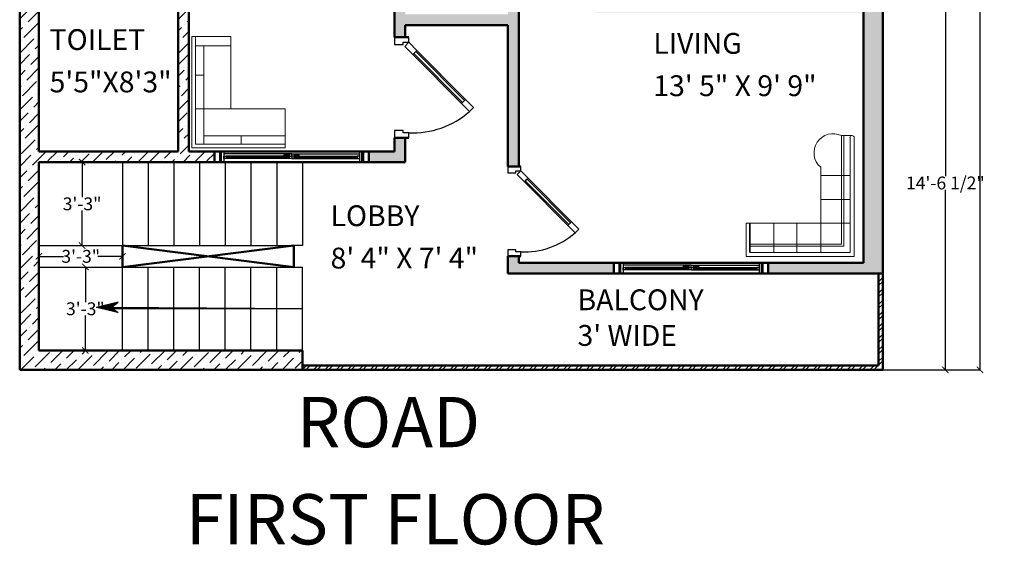
# Model space of a CAD drawing. Units: inches. Extents: x 2278 to 7495, y -71 to 1198.
# Tile 5 of 44: x 2846 to 3306, y 627 to 873. Entities that reach past the tile are written whole.
import ezdxf

# ---------------------------------------------------------------- set-up
doc = ezdxf.new("R2010")
doc.units = ezdxf.units.IN
doc.header["$MEASUREMENT"] = 0
for name, color, linetype, lineweight in [('A-ANNO-DIMS', 2, 'Continuous', 18), ('A-ANNO-TEXT', 7, 'Continuous', 25), ('A-AREA-IDEN', 3, 'Continuous', 18), ('A-Door', 3, 'Continuous', 25), ('A-FLOR-PATT', 252, 'Continuous', 13), ('A-FLOR-STRS', 6, 'Continuous', 25), ('A-FURN', 8, 'Continuous', 18), ('A-Glaz', 4, 'Continuous', 25), ('A-Wall', 7, 'Continuous', 50), ('A-WALL-PATT', 8, 'Continuous', 18)]:
    doc.layers.add(name, color=color, linetype=linetype, lineweight=lineweight)
doc.styles.get("Standard").update_dxf_attribs({"font": 'arial.ttf'})
doc.dimstyles.get("Standard").update_dxf_attribs({"dimtxt": 6, "dimasz": 3, "dimexe": 0.18, "dimexo": 0.0625, "dimgap": 0.09, "dimtad": 0, "dimtih": 1, "dimtoh": 1, "dimdec": 0, "dimzin": 0, "dimdsep": 46, "dimlunit": 3, "dimtxsty": 'Standard', "dimblk": 'ARCHTICK', "dimcen": 0.09, "dimadec": 0, "dimazin": 0, "dimtfac": 1, "dimtdec": 0, "dimtofl": 0, "dimtmove": 0, "dimatfit": 3, "dimfxl": 1, "dimtolj": 1, "dimtzin": 0, "dimarcsym": 0})

# ---------------------------------------------------------------- blocks, each defined once
blk = doc.blocks.new('A$C1DF4181C')
blk.add_lwpolyline([(120, 128), (460.7, 466.1), (432.5, 494.5), (91.8, 156.4)], close=True)
blk.add_arc((72.4, 128.7), 593.3, 357.23132, 41.49368)
at = {"layer": 'A-Door'}
for points in [[(517.5, 522.4), (460.7, 466.1), (432.5, 494.5), (489.3, 550.8)], [(63.2, 71.6), (120, 128), (91.8, 156.4), (35, 100)], [(35, 100), (0, 100), (0, 0), (50, 0), (50, 50), (50, 60), (35, 60)], [(665, 100), (665, 60), (650, 60), (650, 50), (650, 0), (700, 0), (700, 100)]]:
    blk.add_lwpolyline(points, close=True, dxfattribs=at)
at = {"layer": 'A-Glaz'}
blk.add_lwpolyline([(112.9, 135.1), (453.6, 473.2), (439.5, 487.4), (98.8, 149.3)], close=True, dxfattribs=at)
at = {"layer": 'A-Wall'}
for p, q in [((0, 0), (0, 100)), ((0, 100), (0, 0)), ((700, 0), (700, 100)), ((700, 0), (700, 100))]:
    blk.add_line(p, q, dxfattribs=at)
blk = doc.blocks.new('_ArchTick')
at = {"color": 0, "linetype": 'ByBlock', "const_width": 0.15}
blk.add_lwpolyline([(-0.5, -0.5), (0.5, 0.5)], dxfattribs=at)
blk = doc.blocks.new('*D14')
at = {"layer": 'A-ANNO-DIMS', "color": 0, "lineweight": -2, "transparency": 16777216}
for p, q in [((2873.88, 806.26), (2875.25, 806.26)), ((2875.07, 806.26), (2875.07, 789.91)), ((2875.07, 767.26), (2875.07, 783.6)), ((2873.88, 767.26), (2875.25, 767.26))]:
    blk.add_line(p, q, dxfattribs=at)
at = {"layer": 'Defpoints', "color": 0, "transparency": 16777216}
for p in [(2873.82, 806.26), (2873.82, 767.26), (2875.07, 767.26)]:
    blk.add_point(p, dxfattribs=at)
at = {"layer": 'A-ANNO-DIMS', "color": 0, "lineweight": -2, "transparency": 16777216, "xscale": 3, "yscale": 3, "zscale": 3}
for p, rotation in [((2875.07, 806.26), 90), ((2875.07, 767.26), 270)]:
    blk.add_blockref('_ArchTick', p, dxfattribs=dict(at, rotation=rotation))
at = {"layer": 'A-ANNO-DIMS', "color": 0, "transparency": 16777216, "insert": (2875.07, 786.76), "char_height": 6, "attachment_point": 5}
blk.add_mtext('\\A1;3\'-3"', dxfattribs=at)
blk = doc.blocks.new('*D15')
at = {"layer": 'A-ANNO-DIMS', "color": 0, "lineweight": -2, "transparency": 16777216}
for p, q in [((2854.93, 762.24), (2866.37, 762.24)), ((2854.93, 762.19), (2854.93, 762.06)), ((2893.93, 762.24), (2882.49, 762.24)), ((2893.93, 762.19), (2893.93, 762.06))]:
    blk.add_line(p, q, dxfattribs=at)
at = {"layer": 'Defpoints', "color": 0, "transparency": 16777216}
for p in [(2854.93, 762.26), (2893.93, 762.26), (2893.93, 762.24)]:
    blk.add_point(p, dxfattribs=at)
at = {"layer": 'A-ANNO-DIMS', "color": 0, "lineweight": -2, "transparency": 16777216, "xscale": 3, "yscale": 3, "zscale": 3, "rotation": 180}
blk.add_blockref('_ArchTick', (2854.93, 762.24), dxfattribs=at)
at = {"layer": 'A-ANNO-DIMS', "color": 0, "lineweight": -2, "transparency": 16777216, "xscale": 3, "yscale": 3, "zscale": 3}
blk.add_blockref('_ArchTick', (2893.93, 762.24), dxfattribs=at)
at = {"layer": 'A-ANNO-DIMS', "color": 0, "transparency": 16777216, "insert": (2874.43, 762.24), "char_height": 6, "attachment_point": 5}
blk.add_mtext('\\A1;3\'-3"', dxfattribs=at)
blk = doc.blocks.new('*D16')
at = {"layer": 'A-ANNO-DIMS', "color": 0, "lineweight": -2, "transparency": 16777216}
for p, q in [((2875.25, 757.26), (2876.78, 757.26)), ((2876.6, 757.26), (2876.6, 740.91)), ((2876.6, 718.26), (2876.6, 734.6)), ((2875.25, 718.26), (2876.78, 718.26))]:
    blk.add_line(p, q, dxfattribs=at)
at = {"layer": 'Defpoints', "color": 0, "transparency": 16777216}
for p in [(2875.19, 757.26), (2875.19, 718.26), (2876.6, 718.26)]:
    blk.add_point(p, dxfattribs=at)
at = {"layer": 'A-ANNO-DIMS', "color": 0, "lineweight": -2, "transparency": 16777216, "xscale": 3, "yscale": 3, "zscale": 3}
for p, rotation in [((2876.6, 757.26), 90), ((2876.6, 718.26), 270)]:
    blk.add_blockref('_ArchTick', p, dxfattribs=dict(at, rotation=rotation))
at = {"layer": 'A-ANNO-DIMS', "color": 0, "transparency": 16777216, "insert": (2876.6, 737.76), "char_height": 6, "attachment_point": 5}
blk.add_mtext('\\A1;3\'-3"', dxfattribs=at)
blk = doc.blocks.new('*D35')
at = {"layer": 'A-ANNO-DIMS', "color": 0, "lineweight": -2, "transparency": 16777216}
for p, q in [((3248.99, 1162.26), (3294.56, 1162.26)), ((3294.38, 1162.26), (3294.38, 938.91)), ((3294.38, 709.26), (3294.38, 932.6)), ((3248.99, 709.26), (3294.56, 709.26))]:
    blk.add_line(p, q, dxfattribs=at)
at = {"layer": 'Defpoints', "color": 0, "transparency": 16777216}
for p in [(3248.93, 1162.26), (3248.93, 709.26), (3294.38, 709.26)]:
    blk.add_point(p, dxfattribs=at)
at = {"layer": 'A-ANNO-DIMS', "color": 0, "lineweight": -2, "transparency": 16777216, "xscale": 3, "yscale": 3, "zscale": 3}
for p, rotation in [((3294.38, 1162.26), 90), ((3294.38, 709.26), 270)]:
    blk.add_blockref('_ArchTick', p, dxfattribs=dict(at, rotation=rotation))
at = {"layer": 'A-ANNO-DIMS', "color": 0, "transparency": 16777216, "insert": (3294.38, 935.76), "char_height": 6, "attachment_point": 5}
blk.add_mtext('\\A1;37\'-9"', dxfattribs=at)
blk = doc.blocks.new('*D90')
at = {"layer": 'A-ANNO-DIMS', "color": 0, "lineweight": -2, "transparency": 16777216}
for p, q in [((3248.99, 883.76), (3278.36, 883.76)), ((3278.18, 883.76), (3278.18, 799.7)), ((3278.18, 709.26), (3278.18, 793.31)), ((3248.99, 709.26), (3278.36, 709.26))]:
    blk.add_line(p, q, dxfattribs=at)
at = {"layer": 'Defpoints', "color": 0, "transparency": 16777216}
for p in [(3248.93, 883.76), (3248.93, 709.26), (3278.18, 709.26)]:
    blk.add_point(p, dxfattribs=at)
at = {"layer": 'A-ANNO-DIMS', "color": 0, "lineweight": -2, "transparency": 16777216, "xscale": 3, "yscale": 3, "zscale": 3}
for p, rotation in [((3278.18, 883.76), 90), ((3278.18, 709.26), 270)]:
    blk.add_blockref('_ArchTick', p, dxfattribs=dict(at, rotation=rotation))
at = {"layer": 'A-ANNO-DIMS', "color": 0, "transparency": 16777216, "insert": (3278.18, 796.51), "char_height": 6, "attachment_point": 5}
blk.add_mtext('\\A1;14\'-6 1/2"', dxfattribs=at)

msp = doc.modelspace()

# ---------------------------------------------------------------- hatches: boundary and pattern name
at = {"layer": 'A-FLOR-PATT'}
h = msp.add_hatch(dxfattribs=at)
h.set_pattern_fill('ANSI31', color=256)
h.set_pattern_definition([(45, (532.06089, -1.20929), (-0.0883883476, 0.0883883476), [])])
h.paths.add_polyline_path([(2888.65, 738.43), (2891.98, 740.88), (2881.75, 738.43), (2891.98, 735.97)])
at = {"layer": 'A-WALL-PATT', "transparency": 33554687}
h = msp.add_hatch(dxfattribs=at)
h.set_pattern_fill('ANSI36', color=256, scale=30)
h.paths.add_polyline_path([(2854.93, 910.26), (2877.93, 910.26), (2877.93, 915.26), (2854.93, 915.26), (2854.93, 951.26), (2875.18, 951.26), (2875.18, 956.26), (2854.93, 956.26), (2854.93, 1028.26), (2883.93, 1028.26), (2883.93, 1033.26), (2854.93, 1033.26), (2854.93, 1153.26), (2871.93, 1153.26), (2871.93, 1162.26), (2845.93, 1162.26), (2845.93, 709.26), (2977.93, 709.26), (2977.93, 718.26), (2854.93, 718.26), (2854.93, 806.26), (2936.93, 806.26), (2936.93, 811.26), (2924.93, 811.26), (2924.93, 880.26), (2919.93, 880.26), (2919.93, 811.26), (2854.93, 811.26)])
h = msp.add_hatch(dxfattribs=at)
h.set_pattern_fill('ANSI36', color=256, scale=30)
h.paths.add_polyline_path([(3248.93, 883.76), (3239.93, 883.76), (3239.93, 881.26), (3119.93, 881.26), (3119.93, 916.26), (3114.93, 916.26), (3114.93, 876.26), (3239.93, 876.26), (3239.93, 759.26), (3195.43, 759.26), (3195.43, 754.26), (3248.93, 754.26)])
h.paths.add_polyline_path([(3248.93, 963.26), (3239.93, 963.26), (3114.93, 963.26), (3114.93, 952.26), (3119.93, 952.26), (3119.93, 958.26), (3239.93, 958.26), (3239.93, 955.76), (3248.93, 955.76)])
h.paths.add_polyline_path([(3078.93, 1076.26), (3090.93, 1076.26), (3090.93, 1081.26), (3078.93, 1081.26), (3078.93, 1153.26), (3090.93, 1153.26), (3090.93, 1162.26), (3055.93, 1162.26), (3055.93, 1153.26), (3073.93, 1153.26), (3073.93, 1033.26), (3007.93, 1033.26), (3007.93, 1028.26), (3073.93, 1028.26), (3073.93, 942.26), (3073.93, 938.92), (3073.93, 875.26), (3025.93, 875.26), (3025.93, 942.26), (3020.93, 942.26), (3020.93, 870.26), (3020.93, 864.53), (3025.94, 864.53), (3025.94, 870.26), (3073.93, 870.26), (3073.93, 804.26), (3078.93, 804.26)])
h.paths.add_polyline_path([(2983.93, 1162.26), (2943.93, 1162.26), (2943.93, 1153.26), (2960.93, 1153.26), (2960.93, 1033.26), (2960.93, 1028.26), (2965.93, 1028.26), (2965.93, 1153.26), (2983.93, 1153.26)])
h.paths.add_polyline_path([(3149.93, 1162.26), (3114.93, 1162.26), (3114.93, 1153.26), (3126.93, 1153.26), (3126.93, 1081.26), (3120.93, 1081.26), (3120.93, 1076.26), (3131.93, 1076.26), (3131.93, 1153.26), (3149.93, 1153.26)])
h.paths.add_polyline_path([(3248.93, 1162.26), (3221.93, 1162.26), (3221.93, 1153.26), (3239.93, 1153.26), (3239.93, 1040.26), (3126.93, 1040.26), (3126.93, 1035.26), (3239.93, 1035.26), (3248.93, 1035.26)])
h.paths.add_polyline_path([(3123.43, 759.26), (3078.93, 759.26), (3078.93, 762.26), (3073.93, 762.26), (3073.93, 754.26), (3123.43, 754.26)])
h.paths.add_polyline_path([(3025.93, 811.26), (3025.89, 817.61), (3020.93, 817.61), (3020.93, 811.26), (3008.93, 811.26), (3008.93, 806.26), (3025.93, 806.26)], flags=17)
h.paths.add_polyline_path([(2924.93, 1028.26), (2924.93, 1033.26), (2913.93, 1033.26), (2913.93, 1028.26), (2919.93, 1028.26), (2919.93, 956.26), (2899.18, 956.26), (2899.18, 951.26), (2924.93, 951.26)])
h.paths.add_polyline_path([(2924.93, 915.26), (2901.93, 915.26), (2901.93, 910.26), (2924.93, 910.26)])
h.paths.add_polyline_path([(3078.14, 1129.24), (3130.7, 1129.24), (3130.7, 1144.33), (3078.14, 1144.33)], flags=9)
at = {"layer": 'A-WALL-PATT'}
h = msp.add_hatch(dxfattribs=at)
h.set_pattern_fill('ANSI32', color=256, scale=10)
h.set_pattern_definition([(45, (-161.574, -1.2093), (-2.6516504, 2.6516504), []), (45, (-159.806, -1.2093), (-2.6516504, 2.6516504), [])])
h.paths.add_polyline_path([(3248.93, 713.26), (3248.93, 754.26), (3246.93, 754.26), (3246.93, 711.26), (2977.93, 711.26), (2977.93, 709.26), (3248.93, 709.26)])

# ---------------------------------------------------------------- linework, layer by layer
at = {"layer": 'A-FLOR-STRS'}
for p, q in [((2893.93, 806.26), (2893.93, 767.26)), ((2905.93, 806.26), (2905.93, 767.26)), ((2917.93, 806.26), (2917.93, 767.26)), ((2929.93, 806.26), (2929.93, 767.26)), ((2941.93, 806.26), (2941.93, 767.26)), ((2953.93, 806.26), (2953.93, 767.26)), ((2965.93, 806.26), (2965.93, 767.26)), ((2977.93, 806.26), (2977.93, 767.26)), ((2854.93, 767.26), (2973.93, 767.26)), ((2977.93, 767.26), (2973.93, 767.26)), ((2854.93, 757.26), (2977.93, 757.26)), ((2893.93, 718.26), (2893.93, 757.26)), ((2905.93, 718.26), (2905.93, 757.26)), ((2917.93, 718.26), (2917.93, 757.26)), ((2929.93, 718.26), (2929.93, 757.26)), ((2941.93, 718.26), (2941.93, 757.26)), ((2953.93, 718.26), (2953.93, 757.26)), ((2965.93, 718.26), (2965.93, 757.26)), ((2977.93, 718.26), (2977.93, 757.26)), ((2891.98, 740.88), (2881.75, 738.43)), ((2888.65, 738.43), (2891.98, 740.88)), ((2891.98, 735.97), (2881.75, 738.43)), ((2977.93, 737.76), (2888.65, 738.43)), ((2888.65, 738.43), (2891.98, 735.97)), ((2977.93, 737.76), (2889.39, 737.76))]:
    msp.add_line(p, q, dxfattribs=at)
at = {"layer": 'A-FURN'}
for p, q in [((2926.28, 812.89), (2926.28, 864.83)), ((2944.51, 864.83), (2926.28, 864.83)), ((2927.96, 814.58), (2927.96, 864.83)), ((2944.51, 831.13), (2944.51, 864.83)), ((2944.51, 860.61), (2927.96, 860.61)), ((2931.85, 814.58), (2931.85, 860.61)), ((2931.85, 846.84), (2927.96, 846.84)), ((2969.89, 831.13), (2927.96, 831.13)), ((2969.89, 812.89), (2969.89, 831.13)), ((2931.85, 818.46), (2969.89, 818.46)), ((2949.41, 814.58), (2949.41, 818.46)), ((3229.74, 818.61), (3229.74, 767.99)), ((3234.62, 818.61), (3229.74, 818.61)), ((3230.71, 818.61), (3230.71, 767.01)), ((2927.96, 814.58), (2969.89, 814.58)), ((3233.65, 817.63), (3233.65, 764.07)), ((3235.6, 817.63), (3235.6, 762.12)), ((2969.89, 812.89), (2926.28, 812.89)), ((3219.96, 799.93), (3219.96, 803.84)), ((3219.96, 764.07), (3219.96, 799.93)), ((3219.96, 775.16), (3219.96, 799.93)), ((3219.96, 799.93), (3233.65, 799.93)), ((3219.96, 799.93), (3233.65, 799.93)), ((3219.96, 788.85), (3233.65, 788.85)), ((3185.08, 777.76), (3233.65, 777.76)), ((3185.08, 762.12), (3185.08, 777.76)), ((3186.71, 764.07), (3186.71, 777.76)), ((3187.04, 764.07), (3187.04, 777.76)), ((3198.12, 764.07), (3198.12, 777.76)), ((3208.88, 764.07), (3208.88, 777.76)), ((3229.74, 767.99), (3187.04, 767.99)), ((3230.71, 767.01), (3187.04, 767.01)), ((3233.65, 764.07), (3187.04, 764.07)), ((3235.6, 762.12), (3185.08, 762.12))]:
    msp.add_line(p, q, dxfattribs=at)
for centre, radius, start, end in [((3225.77, 810.61), 8.93, 63.5922, 229.3979), ((3234.62, 817.63), 0.978, 0, 180)]:
    msp.add_arc(centre, radius, start, end, dxfattribs=at)
at = {"layer": 'A-Glaz'}
for p, q in [((2972.93, 811.26), (2941.21, 811.26)), ((2972.93, 810.05), (2941.21, 810.05)), ((2971.85, 809.51), (2969.52, 809.51)), ((2972.93, 811.26), (3004.65, 811.26)), ((2972.93, 810.05), (3004.65, 810.05)), ((2974.02, 809.51), (2976.34, 809.51)), ((2972.93, 806.26), (2941.21, 806.26)), ((2971.85, 808.97), (2942.29, 808.97)), ((2971.85, 808.43), (2942.29, 808.43)), ((2971.85, 807.88), (2942.29, 807.88)), ((2972.93, 806.26), (3004.65, 806.26)), ((2974.02, 808.97), (3003.57, 808.97)), ((2974.02, 808.43), (3003.57, 808.43)), ((2974.02, 807.88), (3003.57, 807.88)), ((3159.43, 759.26), (3127.71, 759.26)), ((3159.43, 759.26), (3191.15, 759.26)), ((3159.43, 758.05), (3127.71, 758.05)), ((3159.43, 754.26), (3127.71, 754.26)), ((3158.35, 756.97), (3128.79, 756.97)), ((3158.35, 756.43), (3128.79, 756.43)), ((3158.35, 755.88), (3128.79, 755.88)), ((3158.35, 757.51), (3156.02, 757.51)), ((3159.43, 758.05), (3191.15, 758.05)), ((3159.43, 754.26), (3191.15, 754.26)), ((3160.52, 757.51), (3162.84, 757.51)), ((3160.52, 756.97), (3190.07, 756.97)), ((3160.52, 756.43), (3190.07, 756.43)), ((3160.52, 755.88), (3190.07, 755.88))]:
    msp.add_line(p, q, dxfattribs=at)
for points in [[(2941.21, 806.26), (2940.12, 806.26), (2940.12, 811.26), (2941.21, 811.26)], [(2969.24, 809.51), (2969.52, 809.67), (2969.52, 809.35)], [(2971.85, 808.97), (2972.93, 808.97), (2972.93, 810.05), (2971.85, 810.05)], [(2974.02, 808.97), (2972.93, 808.97), (2972.93, 810.05), (2974.02, 810.05)], [(2976.62, 809.51), (2976.34, 809.67), (2976.34, 809.35)], [(3004.65, 806.26), (3005.74, 806.26), (3005.74, 811.26), (3004.65, 811.26)], [(2942.29, 807.88), (2941.21, 807.88), (2941.21, 808.97), (2942.29, 808.97)], [(2972.93, 807.88), (2971.85, 807.88), (2971.85, 808.97), (2972.93, 808.97)], [(2972.93, 807.88), (2974.02, 807.88), (2974.02, 808.97), (2972.93, 808.97)], [(3003.57, 807.88), (3004.65, 807.88), (3004.65, 808.97), (3003.57, 808.97)], [(3127.71, 754.26), (3126.62, 754.26), (3126.62, 759.26), (3127.71, 759.26)], [(3191.15, 754.26), (3192.24, 754.26), (3192.24, 759.26), (3191.15, 759.26)], [(3128.79, 755.88), (3127.71, 755.88), (3127.71, 756.97), (3128.79, 756.97)], [(3155.74, 757.51), (3156.02, 757.67), (3156.02, 757.35)], [(3158.35, 756.97), (3159.43, 756.97), (3159.43, 758.05), (3158.35, 758.05)], [(3159.43, 755.88), (3158.35, 755.88), (3158.35, 756.97), (3159.43, 756.97)], [(3160.52, 756.97), (3159.43, 756.97), (3159.43, 758.05), (3160.52, 758.05)], [(3159.43, 755.88), (3160.52, 755.88), (3160.52, 756.97), (3159.43, 756.97)], [(3163.12, 757.51), (3162.84, 757.67), (3162.84, 757.35)], [(3190.07, 755.88), (3191.15, 755.88), (3191.15, 756.97), (3190.07, 756.97)]]:
    msp.add_lwpolyline(points, close=True, dxfattribs=at)
at = {"layer": 'A-Wall'}
for p, q in [((2845.93, 1162.26), (2845.93, 709.26)), ((3248.93, 1162.26), (3248.93, 713.26)), ((3078.93, 1076.26), (3078.93, 804.26)), ((3020.93, 942.26), (3020.93, 870.26)), ((2854.93, 910.26), (2854.93, 811.26)), ((2919.93, 880.26), (2919.93, 811.26)), ((2924.93, 880.26), (2924.93, 811.26)), ((3239.93, 876.26), (3239.93, 759.26)), ((3020.93, 870.26), (3020.93, 864.53)), ((3025.93, 870.26), (3073.93, 870.26)), ((3025.94, 864.53), (3025.94, 870.26)), ((3073.93, 870.26), (3073.93, 804.26)), ((3020.93, 864.53), (3025.94, 864.53)), ((3020.93, 811.26), (3020.93, 817.61)), ((3020.93, 817.61), (3025.89, 817.61)), ((3025.89, 817.61), (3025.93, 811.26)), ((2854.93, 811.26), (2919.93, 811.26)), ((2924.93, 811.26), (3020.93, 811.26)), ((2936.93, 806.26), (2936.93, 811.26)), ((2940.12, 811.26), (2936.93, 811.26)), ((2939.58, 811.14), (2939.58, 806.8)), ((3005.74, 811.26), (3008.93, 811.26)), ((3006.28, 811.14), (3006.28, 806.8)), ((3008.93, 806.26), (3008.93, 811.26)), ((3025.93, 811.26), (3025.93, 806.26)), ((2854.93, 806.26), (2854.93, 718.26)), ((2854.93, 806.26), (3025.93, 806.26)), ((2940.12, 806.26), (2936.93, 806.26)), ((3005.74, 806.26), (3008.93, 806.26)), ((3078.93, 804.26), (3073.93, 804.26)), ((2893.93, 757.26), (2893.93, 767.26)), ((2893.93, 757.26), (2973.93, 767.26)), ((2973.93, 757.26), (2893.93, 767.26)), ((2973.93, 767.26), (2973.93, 757.26)), ((3073.93, 762.26), (3073.93, 754.26)), ((3078.93, 762.26), (3073.93, 762.26)), ((3078.93, 762.26), (3078.93, 759.26)), ((3078.93, 759.26), (3239.93, 759.26)), ((3123.43, 754.26), (3123.43, 759.26)), ((3126.62, 759.26), (3123.43, 759.26)), ((3126.08, 759.14), (3126.08, 754.8)), ((3192.24, 759.26), (3195.43, 759.26)), ((3192.78, 759.14), (3192.78, 754.8)), ((3195.43, 754.26), (3195.43, 759.26)), ((3073.93, 754.26), (3248.93, 754.26)), ((3126.62, 754.26), (3123.43, 754.26)), ((3192.24, 754.26), (3195.43, 754.26)), ((3246.93, 754.26), (3246.93, 711.26)), ((2854.93, 718.26), (2977.93, 718.26)), ((2977.93, 709.26), (2977.93, 718.26)), ((3248.93, 709.26), (3248.93, 713.26)), ((2845.93, 709.26), (2977.93, 709.26)), ((2977.93, 711.26), (3246.93, 711.26)), ((2977.93, 709.26), (3248.93, 709.26))]:
    msp.add_line(p, q, dxfattribs=at)

# ---------------------------------------------------------------- block references
at = {"layer": 'A-Door', "rotation": 270}
for p, xscale, yscale, zscale in [((3020.93, 864.53), 0.0670393380383952, 0.0670393380383952, 0.0670393380383952), ((3073.93, 804.26), 0.0599999999999766, 0.0599999999999766, 0.0599999999999766)]:
    msp.add_blockref('A$C1DF4181C', p, dxfattribs=dict(at, xscale=xscale, yscale=yscale, zscale=zscale))

# ---------------------------------------------------------------- texts
at = {"layer": 'A-ANNO-TEXT'}
for s, height, p in [('ROAD', 23.481, (2975.33, 673.11)), ('FIRST FLOOR', 23.4811, (2923.42, 627.72))]:
    msp.add_text(s, height=height, dxfattribs=at).set_placement(p)
at = {"layer": 'A-AREA-IDEN'}
for s, height, p in [('TOILET', 9.72, (2859.9, 858.6)), ('LIVING', 9.72, (3141.8, 856.83)), ('5\'5"X8\'3"', 9.72, (2859.9, 838.83)), ('13\' 5" X 9\' 9"', 9.7203, (3141.8, 837.06)), ('LOBBY', 9.72, (2991.1, 776.35)), ('8\' 4" X 7\' 4"', 9.7203, (2991.1, 756.57)), ('BALCONY ', 9.72, (3106.4, 737.09)), ("3' WIDE", 9.72, (3106.4, 720.45))]:
    msp.add_text(s, height=height, dxfattribs=at).set_placement(p)

# ---------------------------------------------------------------- dimensions: what is measured, and where the dimension line sits
at = {"layer": 'A-ANNO-DIMS'}
for base, p1, p2, override, picture, middle in [((3294.38, 709.26), (3248.93, 1162.26), (3248.93, 709.26), {"dimclrd": 0, "dimclre": 0, "dimclrt": 0}, '*D35', (3294.38, 935.76)), ((3278.18, 709.26), (3248.93, 883.76), (3248.93, 709.26), {"dimdec": 1, "dimlfac": 1, "dimrnd": 0, "dimzin": 1, "dimdsep": 46, "dimlunit": 4, "dimfrac": 2}, '*D90', (3278.18, 796.51)), ((2875.07, 767.26), (2873.82, 806.26), (2873.82, 767.26), {"dimclrd": 0, "dimclre": 0, "dimclrt": 0}, '*D14', (2875.07, 786.76)), ((2876.6, 718.26), (2875.19, 757.26), (2875.19, 718.26), {"dimclrd": 0, "dimclre": 0, "dimclrt": 0}, '*D16', (2876.6, 737.76))]:
    dim = msp.add_linear_dim(base=base, p1=p1, p2=p2, angle=90, dimstyle='Standard', override=override, dxfattribs=at)
    dim.commit()
    dim.dimension.update_dxf_attribs({"geometry": picture, "text_midpoint": middle})
dim = msp.add_linear_dim(base=(2893.93, 762.24), p1=(2854.93, 762.26), p2=(2893.93, 762.26), dimstyle='Standard', override={"dimclrd": 0, "dimclre": 0, "dimclrt": 0}, dxfattribs=at)
dim.commit()
dim.dimension.update_dxf_attribs({"geometry": '*D15', "text_midpoint": (2874.43, 762.24)})

doc.saveas('drawing.dxf')
